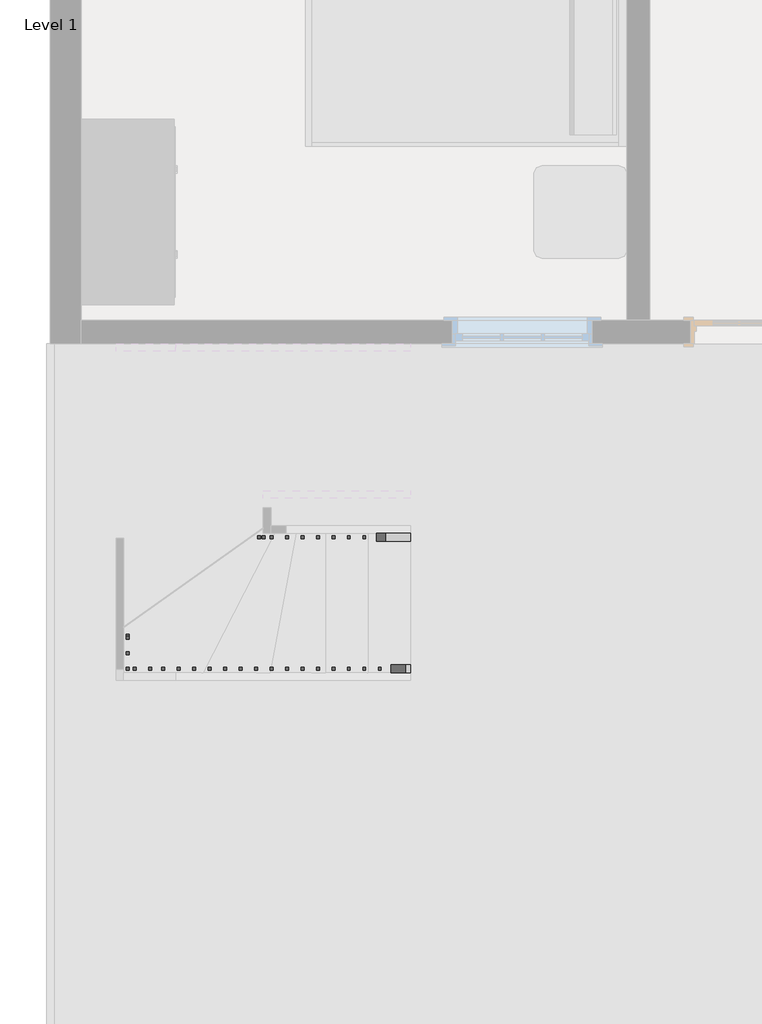
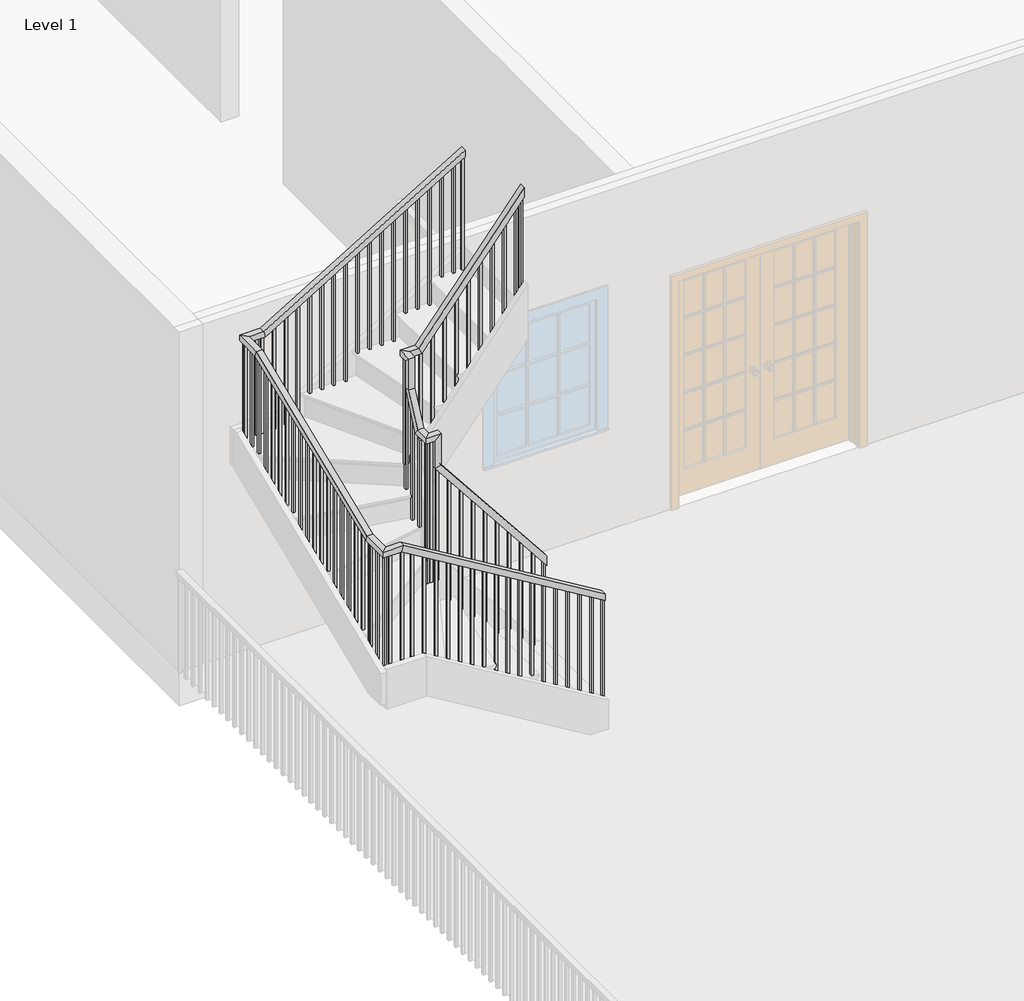
# One storey, part 4 of 5: 2 railings.
"""IFC4 building model written with IfcOpenShell, lengths in millimetres."""

from ifc_helpers import new_model, si_unit, frame, origin, place, context, project, spatial, polyline, outline, extrude, faceted_brep, element, save

model = new_model("IFC4")

# Units and contexts
model_context = context("Model", 3, world=origin())
ifc_project = project(units=[si_unit("LENGTHUNIT", "METRE", prefix="MILLI")], contexts=[model_context])

# Site, building, storey
site = spatial("IfcSite", under=ifc_project)
building = spatial("IfcBuilding", under=site)
storey = spatial("IfcBuildingStorey", under=building, Name="Level 1", Elevation=0.0)

# Railings
placement = place(None, origin())
element("IfcRailing", 1, ObjectType="Handrail - Rectangular", at=placement, inside=storey, context=model_context, shape_type="SolidModel", body=[
    faceted_brep([(-6646.4853347, -3768.8076646, 995.7905875), (-6646.4853347, -3768.8076646, 913.7893268), (-6646.4853347, -3718.0076646, 913.7893268), (-6646.4853347, -3718.0076646, 995.7905875), (-7539.2170266, -3768.8076646, 2127.0036455), (-7590.0170266, -3768.8076646, 2109.3729274), (-7590.0170266, -3718.0076646, 2109.3729274), (-7539.2170266, -3718.0076646, 2127.0036455), (-7539.2170266, -3768.8076646, 2407.836242), (-7590.0170266, -3768.8076646, 2357.036242), (-7590.0170266, -3718.0076646, 2357.036242), (-7539.2170266, -3718.0076646, 2407.836242), (-7666.2170266, -3768.8076646, 2407.836242), (-7666.2170266, -3768.8076646, 2357.036242), (-7615.4170266, -3718.0076646, 2357.036242), (-7615.4170266, -3718.0076646, 2407.836242), (-7666.2170266, -3641.8076646, 2407.836242), (-7666.2170266, -3609.1239512, 2357.036242), (-7615.4170266, -3609.1239512, 2357.036242), (-7615.4170266, -3641.8076646, 2407.836242), (-7666.2170266, -3514.8076646, 2686.6780438), (-7666.2170266, -3464.0076646, 2675.6542485), (-7615.4170266, -3464.0076646, 2675.6542485), (-7615.4170266, -3514.8076646, 2686.6780438), (-7666.2170266, -3514.8076646, 2967.5106402), (-7666.2170266, -3464.0076646, 2916.7106402), (-7615.4170266, -3464.0076646, 2916.7106402), (-7615.4170266, -3514.8076646, 2967.5106402), (-7666.2170266, -3387.8076646, 2967.5106402), (-7666.2170266, -3387.8076646, 2916.7106402), (-7615.4170266, -3438.6076646, 2916.7106402), (-7615.4170266, -3438.6076646, 2967.5106402), (-7539.2170266, -3387.8076646, 2967.5106402), (-7514.5935889, -3387.8076646, 2916.7106402), (-7514.5935889, -3438.6076646, 2916.7106402), (-7539.2170266, -3438.6076646, 2967.5106402), (-6646.4853347, -3387.8076646, 4098.7236983), (-6646.4853347, -3438.6076646, 4098.7236983), (-6646.4853347, -3438.6076646, 4016.7224376), (-6646.4853347, -3387.8076646, 4016.7224376)], [[[0, 1, 2, 3]], [[1, 0, 4, 5]], [[2, 1, 5, 6]], [[3, 2, 6, 7]], [[0, 3, 7, 4]], [[5, 4, 8, 9]], [[6, 5, 9, 10]], [[7, 6, 10, 11]], [[4, 7, 11, 8]], [[9, 8, 12, 13]], [[10, 9, 13, 14]], [[11, 10, 14, 15]], [[8, 11, 15, 12]], [[13, 12, 16, 17]], [[14, 13, 17, 18]], [[15, 14, 18, 19]], [[12, 15, 19, 16]], [[17, 16, 20, 21]], [[18, 17, 21, 22]], [[19, 18, 22, 23]], [[16, 19, 23, 20]], [[21, 20, 24, 25]], [[22, 21, 25, 26]], [[23, 22, 26, 27]], [[20, 23, 27, 24]], [[25, 24, 28, 29]], [[26, 25, 29, 30]], [[27, 26, 30, 31]], [[24, 27, 31, 28]], [[29, 28, 32, 33]], [[30, 29, 33, 34]], [[31, 30, 34, 35]], [[28, 31, 35, 32]], [[36, 37, 38, 39]], [[33, 32, 36, 39]], [[34, 33, 39, 38]], [[35, 34, 38, 37]], [[32, 35, 37, 36]]]),
    extrude(outline(polyline([(3962.998502, -6688.8832363), (3938.8595485, -6707.9332363), (2830.2857143, -6707.9332363), (2830.2857143, -6688.8832363), (3962.998502, -6688.8832363)])), frame((0.0, -3422.7326646, 0.0), z_axis=(0.0, 1.0, 0.0), x_axis=(0.0, 0.0, 1.0)), (0.0, 0.0, 1.0), 19.05),
    extrude(outline(polyline([(3834.2574169, -6790.4832363), (3810.1184634, -6809.5332363), (2830.2857143, -6809.5332363), (2830.2857143, -6790.4832363), (3834.2574169, -6790.4832363)])), frame((0.0, -3422.7326646, 0.0), z_axis=(0.0, 1.0, 0.0), x_axis=(0.0, 0.0, 1.0)), (0.0, 0.0, 1.0), 19.05),
    extrude(outline(polyline([(3705.5163318, -6892.0832363), (3681.3773784, -6911.1332363), (2830.2857143, -6911.1332363), (2830.2857143, -6892.0832363), (3705.5163318, -6892.0832363)])), frame((0.0, -3422.7326646, 0.0), z_axis=(0.0, 1.0, 0.0), x_axis=(0.0, 0.0, 1.0)), (0.0, 0.0, 1.0), 19.05),
    extrude(outline(polyline([(3576.7752467, -6993.6832363), (3552.6362933, -7012.7332363), (2612.5714286, -7012.7332363), (2612.5714286, -6993.6832363), (3576.7752467, -6993.6832363)])), frame((0.0, -3422.7326646, 0.0), z_axis=(0.0, 1.0, 0.0), x_axis=(0.0, 0.0, 1.0)), (0.0, 0.0, 1.0), 19.05),
    extrude(outline(polyline([(3448.0341617, -7095.2832363), (3423.8952082, -7114.3332363), (2612.5714286, -7114.3332363), (2612.5714286, -7095.2832363), (3448.0341617, -7095.2832363)])), frame((0.0, -3422.7326646, 0.0), z_axis=(0.0, 1.0, 0.0), x_axis=(0.0, 0.0, 1.0)), (0.0, 0.0, 1.0), 19.05),
    extrude(outline(polyline([(3319.2930766, -7196.8832363), (3295.1541231, -7215.9332363), (2394.8571429, -7215.9332363), (2394.8571429, -7196.8832363), (3319.2930766, -7196.8832363)])), frame((0.0, -3422.7326646, 0.0), z_axis=(0.0, 1.0, 0.0), x_axis=(0.0, 0.0, 1.0)), (0.0, 0.0, 1.0), 19.05),
    extrude(outline(polyline([(3190.5519915, -7298.4832363), (3166.413038, -7317.5332363), (2394.8571429, -7317.5332363), (2394.8571429, -7298.4832363), (3190.5519915, -7298.4832363)])), frame((0.0, -3422.7326646, 0.0), z_axis=(0.0, 1.0, 0.0), x_axis=(0.0, 0.0, 1.0)), (0.0, 0.0, 1.0), 19.05),
    extrude(outline(polyline([(3061.8109064, -7400.0832363), (3037.671953, -7419.1332363), (2177.1428571, -7419.1332363), (2177.1428571, -7400.0832363), (3061.8109064, -7400.0832363)])), frame((0.0, -3422.7326646, 0.0), z_axis=(0.0, 1.0, 0.0), x_axis=(0.0, 0.0, 1.0)), (0.0, 0.0, 1.0), 19.05),
    extrude(outline(polyline([(2933.0698213, -7501.6832363), (2908.9308679, -7520.7332363), (2177.1428571, -7520.7332363), (2177.1428571, -7501.6832363), (2933.0698213, -7501.6832363)])), frame((0.0, -3422.7326646, 0.0), z_axis=(0.0, 1.0, 0.0), x_axis=(0.0, 0.0, 1.0)), (0.0, 0.0, 1.0), 19.05),
    extrude(outline(polyline([(-3533.5681135, 2522.9269973), (-3514.5181135, 2564.7532676), (-3514.5181135, 1524.0), (-3533.5681135, 1524.0), (-3533.5681135, 2522.9269973)])), frame((-7650.3420266, 0.0, 0.0), z_axis=(1.0, 0.0, 0.0), x_axis=(0.0, 1.0, 0.0)), (0.0, 0.0, 1.0), 19.05),
    extrude(outline(polyline([(-3635.1681135, 2299.8535559), (-3616.1181135, 2341.6798262), (-3616.1181135, 1524.0), (-3635.1681135, 1524.0), (-3635.1681135, 2299.8535559)])), frame((-7650.3420266, 0.0, 0.0), z_axis=(1.0, 0.0, 0.0), x_axis=(0.0, 1.0, 0.0)), (0.0, 0.0, 1.0), 19.05),
    extrude(outline(polyline([(2060.3896158, -7551.3603347), (2084.5285693, -7570.4103347), (1088.5714286, -7570.4103347), (1088.5714286, -7551.3603347), (2060.3896158, -7551.3603347)])), frame((0.0, -3752.9326646, 0.0), z_axis=(0.0, 1.0, 0.0), x_axis=(0.0, 0.0, 1.0)), (0.0, 0.0, 1.0), 19.05),
    extrude(outline(polyline([(1931.6485307, -7449.7603347), (1955.7874842, -7468.8103347), (870.8571429, -7468.8103347), (870.8571429, -7449.7603347), (1931.6485307, -7449.7603347)])), frame((0.0, -3752.9326646, 0.0), z_axis=(0.0, 1.0, 0.0), x_axis=(0.0, 0.0, 1.0)), (0.0, 0.0, 1.0), 19.05),
    extrude(outline(polyline([(1802.9074456, -7348.1603347), (1827.0463991, -7367.2103347), (653.1428571, -7367.2103347), (653.1428571, -7348.1603347), (1802.9074456, -7348.1603347)])), frame((0.0, -3752.9326646, 0.0), z_axis=(0.0, 1.0, 0.0), x_axis=(0.0, 0.0, 1.0)), (0.0, 0.0, 1.0), 19.05),
    extrude(outline(polyline([(1674.1663606, -7246.5603347), (1698.305314, -7265.6103347), (653.1428571, -7265.6103347), (653.1428571, -7246.5603347), (1674.1663606, -7246.5603347)])), frame((0.0, -3752.9326646, 0.0), z_axis=(0.0, 1.0, 0.0), x_axis=(0.0, 0.0, 1.0)), (0.0, 0.0, 1.0), 19.05),
    extrude(outline(polyline([(1545.4252755, -7144.9603347), (1569.5642289, -7164.0103347), (435.4285714, -7164.0103347), (435.4285714, -7144.9603347), (1545.4252755, -7144.9603347)])), frame((0.0, -3752.9326646, 0.0), z_axis=(0.0, 1.0, 0.0), x_axis=(0.0, 0.0, 1.0)), (0.0, 0.0, 1.0), 19.05),
    extrude(outline(polyline([(1416.6841904, -7043.3603347), (1440.8231439, -7062.4103347), (435.4285714, -7062.4103347), (435.4285714, -7043.3603347), (1416.6841904, -7043.3603347)])), frame((0.0, -3752.9326646, 0.0), z_axis=(0.0, 1.0, 0.0), x_axis=(0.0, 0.0, 1.0)), (0.0, 0.0, 1.0), 19.05),
    extrude(outline(polyline([(1287.9431053, -6941.7603347), (1312.0820588, -6960.8103347), (435.4285714, -6960.8103347), (435.4285714, -6941.7603347), (1287.9431053, -6941.7603347)])), frame((0.0, -3752.9326646, 0.0), z_axis=(0.0, 1.0, 0.0), x_axis=(0.0, 0.0, 1.0)), (0.0, 0.0, 1.0), 19.05),
    extrude(outline(polyline([(1159.2020203, -6840.1603347), (1183.3409737, -6859.2103347), (217.7142857, -6859.2103347), (217.7142857, -6840.1603347), (1159.2020203, -6840.1603347)])), frame((0.0, -3752.9326646, 0.0), z_axis=(0.0, 1.0, 0.0), x_axis=(0.0, 0.0, 1.0)), (0.0, 0.0, 1.0), 19.05),
    extrude(outline(polyline([(1030.4609352, -6738.5603347), (1054.5998886, -6757.6103347), (217.7142857, -6757.6103347), (217.7142857, -6738.5603347), (1030.4609352, -6738.5603347)])), frame((0.0, -3752.9326646, 0.0), z_axis=(0.0, 1.0, 0.0), x_axis=(0.0, 0.0, 1.0)), (0.0, 0.0, 1.0), 19.05),
    extrude(outline(polyline([(-7622.3332363, -3422.7326646), (-7622.3332363, -3403.6826646), (-7603.2832363, -3403.6826646), (-7603.2832363, -3422.7326646), (-7622.3332363, -3422.7326646)])), frame((0.0, 0.0, 1959.4285714), z_axis=(0.0, 0.0, 1.0), x_axis=(1.0, 0.0, 0.0)), (0.0, 0.0, 1.0), 957.2820688),
    extrude(outline(polyline([(-7631.2920266, -3422.7326646), (-7650.3420266, -3422.7326646), (-7650.3420266, -3403.6826646), (-7631.2920266, -3403.6826646), (-7631.2920266, -3422.7326646)])), frame((0.0, 0.0, 1959.4285714), z_axis=(0.0, 0.0, 1.0), x_axis=(1.0, 0.0, 0.0)), (0.0, 0.0, 1.0), 957.2820688),
    extrude(outline(polyline([(-7631.2920266, -3438.8972157), (-7650.3420266, -3438.8972157), (-7650.3420266, -3419.8472157), (-7631.2920266, -3419.8472157), (-7631.2920266, -3438.8972157)])), frame((0.0, 0.0, 1741.7142857), z_axis=(0.0, 0.0, 1.0), x_axis=(1.0, 0.0, 0.0)), (0.0, 0.0, 1.0), 1174.9963545),
    extrude(outline(polyline([(-7631.2920266, -3736.7681135), (-7650.3420266, -3736.7681135), (-7650.3420266, -3717.7181135), (-7631.2920266, -3717.7181135), (-7631.2920266, -3736.7681135)])), frame((0.0, 0.0, 1306.2857143), z_axis=(0.0, 0.0, 1.0), x_axis=(1.0, 0.0, 0.0)), (0.0, 0.0, 1.0), 1050.7505277),
    extrude(outline(polyline([(-7631.2920266, -3733.8826646), (-7631.2920266, -3752.9326646), (-7650.3420266, -3752.9326646), (-7650.3420266, -3733.8826646), (-7631.2920266, -3733.8826646)])), frame((0.0, 0.0, 1088.5714286), z_axis=(0.0, 0.0, 1.0), x_axis=(1.0, 0.0, 0.0)), (0.0, 0.0, 1.0), 1268.4648134),
    extrude(outline(polyline([(-7603.2832363, -3733.8826646), (-7603.2832363, -3752.9326646), (-7622.3332363, -3752.9326646), (-7622.3332363, -3733.8826646), (-7603.2832363, -3733.8826646)])), frame((0.0, 0.0, 1088.5714286), z_axis=(0.0, 0.0, 1.0), x_axis=(1.0, 0.0, 0.0)), (0.0, 0.0, 1.0), 1268.4648134),
    extrude(outline(polyline([(4016.7224376, -6646.4853347), (3992.5834842, -6665.5353347), (2830.2857143, -6665.5353347), (2830.2857143, -6646.4853347), (4016.7224376, -6646.4853347)])), frame((0.0, -3422.7326646, 0.0), z_axis=(0.0, 1.0, 0.0), x_axis=(0.0, 0.0, 1.0)), (0.0, 0.0, 1.0), 19.05),
    extrude(outline(polyline([(913.7893268, -6646.4853347), (937.9282803, -6665.5353347), (217.7142857, -6665.5353347), (217.7142857, -6646.4853347), (913.7893268, -6646.4853347)])), frame((0.0, -3752.9326646, 0.0), z_axis=(0.0, 1.0, 0.0), x_axis=(0.0, 0.0, 1.0)), (0.0, 0.0, 1.0), 19.05),
])
element("IfcRailing", 2, ObjectType="Handrail - Rectangular", at=placement, inside=storey, context=model_context, shape_type="SolidModel", body=[
    faceted_brep([(-6646.4853347, -4632.4076646, 1181.4953314), (-6646.4853347, -4632.4076646, 1122.1879128), (-6646.4853347, -4581.6076646, 1122.1879128), (-6646.4853347, -4581.6076646, 1181.4953314), (-8356.6943689, -4632.4076646, 2211.8640781), (-8370.8150071, -4632.4076646, 2161.0640781), (-8370.8150071, -4581.6076646, 2161.0640781), (-8356.6943689, -4581.6076646, 2211.8640781), (-8529.8170266, -4632.4076646, 2211.8640781), (-8529.8170266, -4632.4076646, 2161.0640781), (-8479.0170266, -4581.6076646, 2161.0640781), (-8479.0170266, -4581.6076646, 2211.8640781), (-8529.8170266, -4391.2774717, 2211.8640781), (-8529.8170266, -4381.2101678, 2161.0640781), (-8479.0170266, -4381.2101678, 2161.0640781), (-8479.0170266, -4391.2774717, 2211.8640781), (-8529.8170266, -2765.3378575, 2882.6502076), (-8529.8170266, -2755.2705537, 2831.8502076), (-8479.0170266, -2755.2705537, 2831.8502076), (-8479.0170266, -2765.3378575, 2882.6502076), (-8529.8170266, -2524.2076646, 2882.6502076), (-8529.8170266, -2524.2076646, 2831.8502076), (-8479.0170266, -2575.0076646, 2831.8502076), (-8479.0170266, -2575.0076646, 2882.6502076), (-8356.6943689, -2524.2076646, 2882.6502076), (-8342.5737308, -2524.2076646, 2831.8502076), (-8342.5737308, -2575.0076646, 2831.8502076), (-8356.6943689, -2575.0076646, 2882.6502076), (-6646.4853347, -2524.2076646, 3913.0189543), (-6646.4853347, -2575.0076646, 3913.0189543), (-6646.4853347, -2575.0076646, 3853.7115356), (-6646.4853347, -2524.2076646, 3853.7115356)], [[[0, 1, 2, 3]], [[1, 0, 4, 5]], [[2, 1, 5, 6]], [[3, 2, 6, 7]], [[0, 3, 7, 4]], [[5, 4, 8, 9]], [[6, 5, 9, 10]], [[7, 6, 10, 11]], [[4, 7, 11, 8]], [[9, 8, 12, 13]], [[10, 9, 13, 14]], [[11, 10, 14, 15]], [[8, 11, 15, 12]], [[13, 12, 16, 17]], [[14, 13, 17, 18]], [[15, 14, 18, 19]], [[12, 15, 19, 16]], [[17, 16, 20, 21]], [[18, 17, 21, 22]], [[19, 18, 22, 23]], [[16, 19, 23, 20]], [[21, 20, 24, 25]], [[22, 21, 25, 26]], [[23, 22, 26, 27]], [[20, 23, 27, 24]], [[28, 29, 30, 31]], [[25, 24, 28, 31]], [[26, 25, 31, 30]], [[27, 26, 30, 29]], [[24, 27, 29, 28]]]),
    extrude(outline(polyline([(3796.9975522, -6740.6193689), (2830.2857143, -6740.6193689), (2830.2857143, -6721.5693689), (3808.4748186, -6721.5693689), (3796.9975522, -6740.6193689)])), frame((0.0, -2559.1326646, 0.0), z_axis=(0.0, 1.0, 0.0), x_axis=(0.0, 0.0, 1.0)), (0.0, 0.0, 1.0), 19.05),
    extrude(outline(polyline([(3735.7854649, -6842.2193689), (2830.2857143, -6842.2193689), (2830.2857143, -6823.1693689), (3747.2627313, -6823.1693689), (3735.7854649, -6842.2193689)])), frame((0.0, -2559.1326646, 0.0), z_axis=(0.0, 1.0, 0.0), x_axis=(0.0, 0.0, 1.0)), (0.0, 0.0, 1.0), 19.05),
    extrude(outline(polyline([(3674.5733777, -6943.8193689), (2612.5714286, -6943.8193689), (2612.5714286, -6924.7693689), (3686.050644, -6924.7693689), (3674.5733777, -6943.8193689)])), frame((0.0, -2559.1326646, 0.0), z_axis=(0.0, 1.0, 0.0), x_axis=(0.0, 0.0, 1.0)), (0.0, 0.0, 1.0), 19.05),
    extrude(outline(polyline([(3613.3612904, -7045.4193689), (2612.5714286, -7045.4193689), (2612.5714286, -7026.3693689), (3624.8385567, -7026.3693689), (3613.3612904, -7045.4193689)])), frame((0.0, -2559.1326646, 0.0), z_axis=(0.0, 1.0, 0.0), x_axis=(0.0, 0.0, 1.0)), (0.0, 0.0, 1.0), 19.05),
    extrude(outline(polyline([(3552.1492031, -7147.0193689), (2612.5714286, -7147.0193689), (2612.5714286, -7127.9693689), (3563.6264695, -7127.9693689), (3552.1492031, -7147.0193689)])), frame((0.0, -2559.1326646, 0.0), z_axis=(0.0, 1.0, 0.0), x_axis=(0.0, 0.0, 1.0)), (0.0, 0.0, 1.0), 19.05),
    extrude(outline(polyline([(3490.9371158, -7248.6193689), (2394.8571429, -7248.6193689), (2394.8571429, -7229.5693689), (3502.4143822, -7229.5693689), (3490.9371158, -7248.6193689)])), frame((0.0, -2559.1326646, 0.0), z_axis=(0.0, 1.0, 0.0), x_axis=(0.0, 0.0, 1.0)), (0.0, 0.0, 1.0), 19.05),
    extrude(outline(polyline([(3429.7250285, -7350.2193689), (2394.8571429, -7350.2193689), (2394.8571429, -7331.1693689), (3441.2022949, -7331.1693689), (3429.7250285, -7350.2193689)])), frame((0.0, -2559.1326646, 0.0), z_axis=(0.0, 1.0, 0.0), x_axis=(0.0, 0.0, 1.0)), (0.0, 0.0, 1.0), 19.05),
    extrude(outline(polyline([(3368.5129413, -7451.8193689), (2394.8571429, -7451.8193689), (2394.8571429, -7432.7693689), (3379.9902076, -7432.7693689), (3368.5129413, -7451.8193689)])), frame((0.0, -2559.1326646, 0.0), z_axis=(0.0, 1.0, 0.0), x_axis=(0.0, 0.0, 1.0)), (0.0, 0.0, 1.0), 19.05),
    extrude(outline(polyline([(3307.300854, -7553.4193689), (2394.8571429, -7553.4193689), (2394.8571429, -7534.3693689), (3318.7781204, -7534.3693689), (3307.300854, -7553.4193689)])), frame((0.0, -2559.1326646, 0.0), z_axis=(0.0, 1.0, 0.0), x_axis=(0.0, 0.0, 1.0)), (0.0, 0.0, 1.0), 19.05),
    extrude(outline(polyline([(3246.0887667, -7655.0193689), (2177.1428571, -7655.0193689), (2177.1428571, -7635.9693689), (3257.5660331, -7635.9693689), (3246.0887667, -7655.0193689)])), frame((0.0, -2559.1326646, 0.0), z_axis=(0.0, 1.0, 0.0), x_axis=(0.0, 0.0, 1.0)), (0.0, 0.0, 1.0), 19.05),
    extrude(outline(polyline([(3184.8766794, -7756.6193689), (2177.1428571, -7756.6193689), (2177.1428571, -7737.5693689), (3196.3539458, -7737.5693689), (3184.8766794, -7756.6193689)])), frame((0.0, -2559.1326646, 0.0), z_axis=(0.0, 1.0, 0.0), x_axis=(0.0, 0.0, 1.0)), (0.0, 0.0, 1.0), 19.05),
    extrude(outline(polyline([(3123.6645922, -7858.2193689), (2177.1428571, -7858.2193689), (2177.1428571, -7839.1693689), (3135.1418585, -7839.1693689), (3123.6645922, -7858.2193689)])), frame((0.0, -2559.1326646, 0.0), z_axis=(0.0, 1.0, 0.0), x_axis=(0.0, 0.0, 1.0)), (0.0, 0.0, 1.0), 19.05),
    extrude(outline(polyline([(3062.4525049, -7959.8193689), (2177.1428571, -7959.8193689), (2177.1428571, -7940.7693689), (3073.9297712, -7940.7693689), (3062.4525049, -7959.8193689)])), frame((0.0, -2559.1326646, 0.0), z_axis=(0.0, 1.0, 0.0), x_axis=(0.0, 0.0, 1.0)), (0.0, 0.0, 1.0), 19.05),
    extrude(outline(polyline([(3001.2404176, -8061.4193689), (1959.4285714, -8061.4193689), (1959.4285714, -8042.3693689), (3012.717684, -8042.3693689), (3001.2404176, -8061.4193689)])), frame((0.0, -2559.1326646, 0.0), z_axis=(0.0, 1.0, 0.0), x_axis=(0.0, 0.0, 1.0)), (0.0, 0.0, 1.0), 19.05),
    extrude(outline(polyline([(2940.0283303, -8163.0193689), (1959.4285714, -8163.0193689), (1959.4285714, -8143.9693689), (2951.5055967, -8143.9693689), (2940.0283303, -8163.0193689)])), frame((0.0, -2559.1326646, 0.0), z_axis=(0.0, 1.0, 0.0), x_axis=(0.0, 0.0, 1.0)), (0.0, 0.0, 1.0), 19.05),
    extrude(outline(polyline([(2878.816243, -8264.6193689), (1959.4285714, -8264.6193689), (1959.4285714, -8245.5693689), (2890.2935094, -8245.5693689), (2878.816243, -8264.6193689)])), frame((0.0, -2559.1326646, 0.0), z_axis=(0.0, 1.0, 0.0), x_axis=(0.0, 0.0, 1.0)), (0.0, 0.0, 1.0), 19.05),
    extrude(outline(polyline([(-8412.3420266, -2540.0826646), (-8393.2920266, -2540.0826646), (-8393.2920266, -2559.1326646), (-8412.3420266, -2559.1326646), (-8412.3420266, -2540.0826646)])), frame((0.0, 0.0, 1959.4285714), z_axis=(0.0, 0.0, 1.0), x_axis=(1.0, 0.0, 0.0)), (0.0, 0.0, 1.0), 872.4216362),
    extrude(outline(polyline([(-8513.9420266, -2571.6628575), (-8513.9420266, -2552.6128575), (-8494.8920266, -2552.6128575), (-8494.8920266, -2571.6628575), (-8513.9420266, -2571.6628575)])), frame((0.0, 0.0, 1959.4285714), z_axis=(0.0, 0.0, 1.0), x_axis=(1.0, 0.0, 0.0)), (0.0, 0.0, 1.0), 872.4216362),
    extrude(outline(polyline([(-8513.9420266, -2673.2628575), (-8513.9420266, -2654.2128575), (-8494.8920266, -2654.2128575), (-8494.8920266, -2673.2628575), (-8513.9420266, -2673.2628575)])), frame((0.0, 0.0, 1959.4285714), z_axis=(0.0, 0.0, 1.0), x_axis=(1.0, 0.0, 0.0)), (0.0, 0.0, 1.0), 872.4216362),
    extrude(outline(polyline([(-2756.1524717, 2831.6264786), (-2756.1524717, 1959.4285714), (-2775.2024717, 1959.4285714), (-2775.2024717, 2823.7673455), (-2756.1524717, 2831.6264786)])), frame((-8513.9420266, 0.0, 0.0), z_axis=(1.0, 0.0, 0.0), x_axis=(0.0, 1.0, 0.0)), (0.0, 0.0, 1.0), 19.05),
    extrude(outline(polyline([(-2857.7524717, 2789.5709935), (-2857.7524717, 1741.7142857), (-2876.8024717, 1741.7142857), (-2876.8024717, 2781.7118604), (-2857.7524717, 2789.5709935)])), frame((-8513.9420266, 0.0, 0.0), z_axis=(1.0, 0.0, 0.0), x_axis=(0.0, 1.0, 0.0)), (0.0, 0.0, 1.0), 19.05),
    extrude(outline(polyline([(-2959.3524717, 2747.6556172), (-2959.3524717, 1741.7142857), (-2978.4024717, 1741.7142857), (-2978.4024717, 2739.7964841), (-2959.3524717, 2747.6556172)])), frame((-8513.9420266, 0.0, 0.0), z_axis=(1.0, 0.0, 0.0), x_axis=(0.0, 1.0, 0.0)), (0.0, 0.0, 1.0), 19.05),
    extrude(outline(polyline([(-3060.9524717, 2705.7402409), (-3060.9524717, 1741.7142857), (-3080.0024717, 1741.7142857), (-3080.0024717, 2697.8811078), (-3060.9524717, 2705.7402409)])), frame((-8513.9420266, 0.0, 0.0), z_axis=(1.0, 0.0, 0.0), x_axis=(0.0, 1.0, 0.0)), (0.0, 0.0, 1.0), 19.05),
    extrude(outline(polyline([(-3162.5524717, 2663.8248646), (-3162.5524717, 1741.7142857), (-3181.6024717, 1741.7142857), (-3181.6024717, 2655.9657315), (-3162.5524717, 2663.8248646)])), frame((-8513.9420266, 0.0, 0.0), z_axis=(1.0, 0.0, 0.0), x_axis=(0.0, 1.0, 0.0)), (0.0, 0.0, 1.0), 19.05),
    extrude(outline(polyline([(-3264.1524717, 2621.9094883), (-3264.1524717, 1741.7142857), (-3283.2024717, 1741.7142857), (-3283.2024717, 2614.0503552), (-3264.1524717, 2621.9094883)])), frame((-8513.9420266, 0.0, 0.0), z_axis=(1.0, 0.0, 0.0), x_axis=(0.0, 1.0, 0.0)), (0.0, 0.0, 1.0), 19.05),
    extrude(outline(polyline([(-3365.7524717, 2579.994112), (-3365.7524717, 1524.0), (-3384.8024717, 1524.0), (-3384.8024717, 2572.1349789), (-3365.7524717, 2579.994112)])), frame((-8513.9420266, 0.0, 0.0), z_axis=(1.0, 0.0, 0.0), x_axis=(0.0, 1.0, 0.0)), (0.0, 0.0, 1.0), 19.05),
    extrude(outline(polyline([(-3467.3524717, 2538.0787357), (-3467.3524717, 1524.0), (-3486.4024717, 1524.0), (-3486.4024717, 2530.2196027), (-3467.3524717, 2538.0787357)])), frame((-8513.9420266, 0.0, 0.0), z_axis=(1.0, 0.0, 0.0), x_axis=(0.0, 1.0, 0.0)), (0.0, 0.0, 1.0), 19.05),
    extrude(outline(polyline([(-3568.9524717, 2496.1633594), (-3568.9524717, 1524.0), (-3588.0024717, 1524.0), (-3588.0024717, 2488.3042264), (-3568.9524717, 2496.1633594)])), frame((-8513.9420266, 0.0, 0.0), z_axis=(1.0, 0.0, 0.0), x_axis=(0.0, 1.0, 0.0)), (0.0, 0.0, 1.0), 19.05),
    extrude(outline(polyline([(-3670.5524717, 2454.2479831), (-3670.5524717, 1524.0), (-3689.6024717, 1524.0), (-3689.6024717, 2446.3888501), (-3670.5524717, 2454.2479831)])), frame((-8513.9420266, 0.0, 0.0), z_axis=(1.0, 0.0, 0.0), x_axis=(0.0, 1.0, 0.0)), (0.0, 0.0, 1.0), 19.05),
    extrude(outline(polyline([(-3772.1524717, 2412.3326068), (-3772.1524717, 1524.0), (-3791.2024717, 1524.0), (-3791.2024717, 2404.4734738), (-3772.1524717, 2412.3326068)])), frame((-8513.9420266, 0.0, 0.0), z_axis=(1.0, 0.0, 0.0), x_axis=(0.0, 1.0, 0.0)), (0.0, 0.0, 1.0), 19.05),
    extrude(outline(polyline([(-3873.7524717, 2370.4172305), (-3873.7524717, 1306.2857143), (-3892.8024717, 1306.2857143), (-3892.8024717, 2362.5580975), (-3873.7524717, 2370.4172305)])), frame((-8513.9420266, 0.0, 0.0), z_axis=(1.0, 0.0, 0.0), x_axis=(0.0, 1.0, 0.0)), (0.0, 0.0, 1.0), 19.05),
    extrude(outline(polyline([(-3975.3524717, 2328.5018542), (-3975.3524717, 1306.2857143), (-3994.4024717, 1306.2857143), (-3994.4024717, 2320.6427212), (-3975.3524717, 2328.5018542)])), frame((-8513.9420266, 0.0, 0.0), z_axis=(1.0, 0.0, 0.0), x_axis=(0.0, 1.0, 0.0)), (0.0, 0.0, 1.0), 19.05),
    extrude(outline(polyline([(-4076.9524717, 2286.586478), (-4076.9524717, 1306.2857143), (-4096.0024717, 1306.2857143), (-4096.0024717, 2278.7273449), (-4076.9524717, 2286.586478)])), frame((-8513.9420266, 0.0, 0.0), z_axis=(1.0, 0.0, 0.0), x_axis=(0.0, 1.0, 0.0)), (0.0, 0.0, 1.0), 19.05),
    extrude(outline(polyline([(-4178.5524717, 2244.6711017), (-4178.5524717, 1306.2857143), (-4197.6024717, 1306.2857143), (-4197.6024717, 2236.8119686), (-4178.5524717, 2244.6711017)])), frame((-8513.9420266, 0.0, 0.0), z_axis=(1.0, 0.0, 0.0), x_axis=(0.0, 1.0, 0.0)), (0.0, 0.0, 1.0), 19.05),
    extrude(outline(polyline([(-4280.1524717, 2202.7557254), (-4280.1524717, 1306.2857143), (-4299.2024717, 1306.2857143), (-4299.2024717, 2194.8965923), (-4280.1524717, 2202.7557254)])), frame((-8513.9420266, 0.0, 0.0), z_axis=(1.0, 0.0, 0.0), x_axis=(0.0, 1.0, 0.0)), (0.0, 0.0, 1.0), 19.05),
    extrude(outline(polyline([(-8513.9420266, -4413.3326646), (-8513.9420266, -4394.2826646), (-8494.8920266, -4394.2826646), (-8494.8920266, -4413.3326646), (-8513.9420266, -4413.3326646)])), frame((0.0, 0.0, 1088.5714286), z_axis=(0.0, 0.0, 1.0), x_axis=(1.0, 0.0, 0.0)), (0.0, 0.0, 1.0), 1072.4926495),
    extrude(outline(polyline([(-8513.9420266, -4514.9326646), (-8513.9420266, -4495.8826646), (-8494.8920266, -4495.8826646), (-8494.8920266, -4514.9326646), (-8513.9420266, -4514.9326646)])), frame((0.0, 0.0, 1088.5714286), z_axis=(0.0, 0.0, 1.0), x_axis=(1.0, 0.0, 0.0)), (0.0, 0.0, 1.0), 1072.4926495),
    extrude(outline(polyline([(-8448.7693689, -4616.5326646), (-8467.8193689, -4616.5326646), (-8467.8193689, -4597.4826646), (-8448.7693689, -4597.4826646), (-8448.7693689, -4616.5326646)])), frame((0.0, 0.0, 1088.5714286), z_axis=(0.0, 0.0, 1.0), x_axis=(1.0, 0.0, 0.0)), (0.0, 0.0, 1.0), 1072.4926495),
    extrude(outline(polyline([(2107.3199424, -8281.6103347), (1088.5714286, -8281.6103347), (1088.5714286, -8262.5603347), (2095.842676, -8262.5603347), (2107.3199424, -8281.6103347)])), frame((0.0, -4616.5326646, 0.0), z_axis=(0.0, 1.0, 0.0), x_axis=(0.0, 0.0, 1.0)), (0.0, 0.0, 1.0), 19.05),
    extrude(outline(polyline([(2046.1078551, -8180.0103347), (1088.5714286, -8180.0103347), (1088.5714286, -8160.9603347), (2034.6305887, -8160.9603347), (2046.1078551, -8180.0103347)])), frame((0.0, -4616.5326646, 0.0), z_axis=(0.0, 1.0, 0.0), x_axis=(0.0, 0.0, 1.0)), (0.0, 0.0, 1.0), 19.05),
    extrude(outline(polyline([(1984.8957678, -8078.4103347), (1088.5714286, -8078.4103347), (1088.5714286, -8059.3603347), (1973.4185015, -8059.3603347), (1984.8957678, -8078.4103347)])), frame((0.0, -4616.5326646, 0.0), z_axis=(0.0, 1.0, 0.0), x_axis=(0.0, 0.0, 1.0)), (0.0, 0.0, 1.0), 19.05),
    extrude(outline(polyline([(1923.6836806, -7976.8103347), (870.8571429, -7976.8103347), (870.8571429, -7957.7603347), (1912.2064142, -7957.7603347), (1923.6836806, -7976.8103347)])), frame((0.0, -4616.5326646, 0.0), z_axis=(0.0, 1.0, 0.0), x_axis=(0.0, 0.0, 1.0)), (0.0, 0.0, 1.0), 19.05),
    extrude(outline(polyline([(1862.4715933, -7875.2103347), (870.8571429, -7875.2103347), (870.8571429, -7856.1603347), (1850.9943269, -7856.1603347), (1862.4715933, -7875.2103347)])), frame((0.0, -4616.5326646, 0.0), z_axis=(0.0, 1.0, 0.0), x_axis=(0.0, 0.0, 1.0)), (0.0, 0.0, 1.0), 19.05),
    extrude(outline(polyline([(1801.259506, -7773.6103347), (870.8571429, -7773.6103347), (870.8571429, -7754.5603347), (1789.7822396, -7754.5603347), (1801.259506, -7773.6103347)])), frame((0.0, -4616.5326646, 0.0), z_axis=(0.0, 1.0, 0.0), x_axis=(0.0, 0.0, 1.0)), (0.0, 0.0, 1.0), 19.05),
    extrude(outline(polyline([(1740.0474187, -7672.0103347), (870.8571429, -7672.0103347), (870.8571429, -7652.9603347), (1728.5701524, -7652.9603347), (1740.0474187, -7672.0103347)])), frame((0.0, -4616.5326646, 0.0), z_axis=(0.0, 1.0, 0.0), x_axis=(0.0, 0.0, 1.0)), (0.0, 0.0, 1.0), 19.05),
    extrude(outline(polyline([(1678.8353314, -7570.4103347), (653.1428571, -7570.4103347), (653.1428571, -7551.3603347), (1667.3580651, -7551.3603347), (1678.8353314, -7570.4103347)])), frame((0.0, -4616.5326646, 0.0), z_axis=(0.0, 1.0, 0.0), x_axis=(0.0, 0.0, 1.0)), (0.0, 0.0, 1.0), 19.05),
    extrude(outline(polyline([(1617.6232442, -7468.8103347), (653.1428571, -7468.8103347), (653.1428571, -7449.7603347), (1606.1459778, -7449.7603347), (1617.6232442, -7468.8103347)])), frame((0.0, -4616.5326646, 0.0), z_axis=(0.0, 1.0, 0.0), x_axis=(0.0, 0.0, 1.0)), (0.0, 0.0, 1.0), 19.05),
    extrude(outline(polyline([(1556.4111569, -7367.2103347), (653.1428571, -7367.2103347), (653.1428571, -7348.1603347), (1544.9338905, -7348.1603347), (1556.4111569, -7367.2103347)])), frame((0.0, -4616.5326646, 0.0), z_axis=(0.0, 1.0, 0.0), x_axis=(0.0, 0.0, 1.0)), (0.0, 0.0, 1.0), 19.05),
    extrude(outline(polyline([(1495.1990696, -7265.6103347), (653.1428571, -7265.6103347), (653.1428571, -7246.5603347), (1483.7218032, -7246.5603347), (1495.1990696, -7265.6103347)])), frame((0.0, -4616.5326646, 0.0), z_axis=(0.0, 1.0, 0.0), x_axis=(0.0, 0.0, 1.0)), (0.0, 0.0, 1.0), 19.05),
    extrude(outline(polyline([(1433.9869823, -7164.0103347), (435.4285714, -7164.0103347), (435.4285714, -7144.9603347), (1422.509716, -7144.9603347), (1433.9869823, -7164.0103347)])), frame((0.0, -4616.5326646, 0.0), z_axis=(0.0, 1.0, 0.0), x_axis=(0.0, 0.0, 1.0)), (0.0, 0.0, 1.0), 19.05),
    extrude(outline(polyline([(1372.7748951, -7062.4103347), (435.4285714, -7062.4103347), (435.4285714, -7043.3603347), (1361.2976287, -7043.3603347), (1372.7748951, -7062.4103347)])), frame((0.0, -4616.5326646, 0.0), z_axis=(0.0, 1.0, 0.0), x_axis=(0.0, 0.0, 1.0)), (0.0, 0.0, 1.0), 19.05),
    extrude(outline(polyline([(1311.5628078, -6960.8103347), (435.4285714, -6960.8103347), (435.4285714, -6941.7603347), (1300.0855414, -6941.7603347), (1311.5628078, -6960.8103347)])), frame((0.0, -4616.5326646, 0.0), z_axis=(0.0, 1.0, 0.0), x_axis=(0.0, 0.0, 1.0)), (0.0, 0.0, 1.0), 19.05),
    extrude(outline(polyline([(1250.3507205, -6859.2103347), (217.7142857, -6859.2103347), (217.7142857, -6840.1603347), (1238.8734541, -6840.1603347), (1250.3507205, -6859.2103347)])), frame((0.0, -4616.5326646, 0.0), z_axis=(0.0, 1.0, 0.0), x_axis=(0.0, 0.0, 1.0)), (0.0, 0.0, 1.0), 19.05),
    extrude(outline(polyline([(1189.1386332, -6757.6103347), (217.7142857, -6757.6103347), (217.7142857, -6738.5603347), (1177.6613669, -6738.5603347), (1189.1386332, -6757.6103347)])), frame((0.0, -4616.5326646, 0.0), z_axis=(0.0, 1.0, 0.0), x_axis=(0.0, 0.0, 1.0)), (0.0, 0.0, 1.0), 19.05),
    extrude(outline(polyline([(-8366.2193689, -2540.0826646), (-8347.1693689, -2540.0826646), (-8347.1693689, -2559.1326646), (-8366.2193689, -2559.1326646), (-8366.2193689, -2540.0826646)])), frame((0.0, 0.0, 1959.4285714), z_axis=(0.0, 0.0, 1.0), x_axis=(1.0, 0.0, 0.0)), (0.0, 0.0, 1.0), 872.4216362),
    extrude(outline(polyline([(-8513.9420266, -2559.1326646), (-8513.9420266, -2540.0826646), (-8494.8920266, -2540.0826646), (-8494.8920266, -2559.1326646), (-8513.9420266, -2559.1326646)])), frame((0.0, 0.0, 1959.4285714), z_axis=(0.0, 0.0, 1.0), x_axis=(1.0, 0.0, 0.0)), (0.0, 0.0, 1.0), 872.4216362),
    extrude(outline(polyline([(-2755.8128575, 2831.6264786), (-2755.8128575, 1959.4285714), (-2774.8628575, 1959.4285714), (-2774.8628575, 2823.7673455), (-2755.8128575, 2831.6264786)])), frame((-8513.9420266, 0.0, 0.0), z_axis=(1.0, 0.0, 0.0), x_axis=(0.0, 1.0, 0.0)), (0.0, 0.0, 1.0), 19.05),
    extrude(outline(polyline([(-8513.9420266, -4400.8024717), (-8513.9420266, -4381.7524717), (-8494.8920266, -4381.7524717), (-8494.8920266, -4400.8024717), (-8513.9420266, -4400.8024717)])), frame((0.0, 0.0, 1088.5714286), z_axis=(0.0, 0.0, 1.0), x_axis=(1.0, 0.0, 0.0)), (0.0, 0.0, 1.0), 1072.4926495),
    extrude(outline(polyline([(-8494.8920266, -4616.5326646), (-8513.9420266, -4616.5326646), (-8513.9420266, -4597.4826646), (-8494.8920266, -4597.4826646), (-8494.8920266, -4616.5326646)])), frame((0.0, 0.0, 1088.5714286), z_axis=(0.0, 0.0, 1.0), x_axis=(1.0, 0.0, 0.0)), (0.0, 0.0, 1.0), 1072.4926495),
    extrude(outline(polyline([(2158.2952926, -8366.2193689), (1088.5714286, -8366.2193689), (1088.5714286, -8347.1693689), (2146.8180263, -8347.1693689), (2158.2952926, -8366.2193689)])), frame((0.0, -4616.5326646, 0.0), z_axis=(0.0, 1.0, 0.0), x_axis=(0.0, 0.0, 1.0)), (0.0, 0.0, 1.0), 19.05),
    extrude(outline(polyline([(3842.2342693, -6665.5353347), (2830.2857143, -6665.5353347), (2830.2857143, -6646.4853347), (3853.7115356, -6646.4853347), (3842.2342693, -6665.5353347)])), frame((0.0, -2559.1326646, 0.0), z_axis=(0.0, 1.0, 0.0), x_axis=(0.0, 0.0, 1.0)), (0.0, 0.0, 1.0), 19.05),
    extrude(outline(polyline([(1133.6651791, -6665.5353347), (217.7142857, -6665.5353347), (217.7142857, -6646.4853347), (1122.1879128, -6646.4853347), (1133.6651791, -6665.5353347)])), frame((0.0, -4616.5326646, 0.0), z_axis=(0.0, 1.0, 0.0), x_axis=(0.0, 0.0, 1.0)), (0.0, 0.0, 1.0), 19.05),
])

save(model, "model.ifc")

# Revit data of these elements
# Type "Handrail - Rectangular"
#   Assembly Code = "C2010400"
#   built-in parameter 1008612 = 0.0416667 (stored number, unit not read)
#   built-in parameter 1008611 = 0.0416667 (stored number, unit not read)
#   built-in parameter 1008609 = 0.333333 (stored number, unit not read)
#   built-in parameter 1008604 = 0.166667 (stored number, unit not read)
#   built-in parameter 1008603 = 0.166667 (stored number, unit not read)
#   Railing Height = 3' - 0"
#   built-in parameter 1008630 = 2
#   built-in parameter 1008610 = 2
#   built-in parameter 1008618 = Baluster - Square : 3/4"
# Elements 1, 2 (IfcRailing, "Handrail - Rectangular")
#   Phase Created = New Construction
